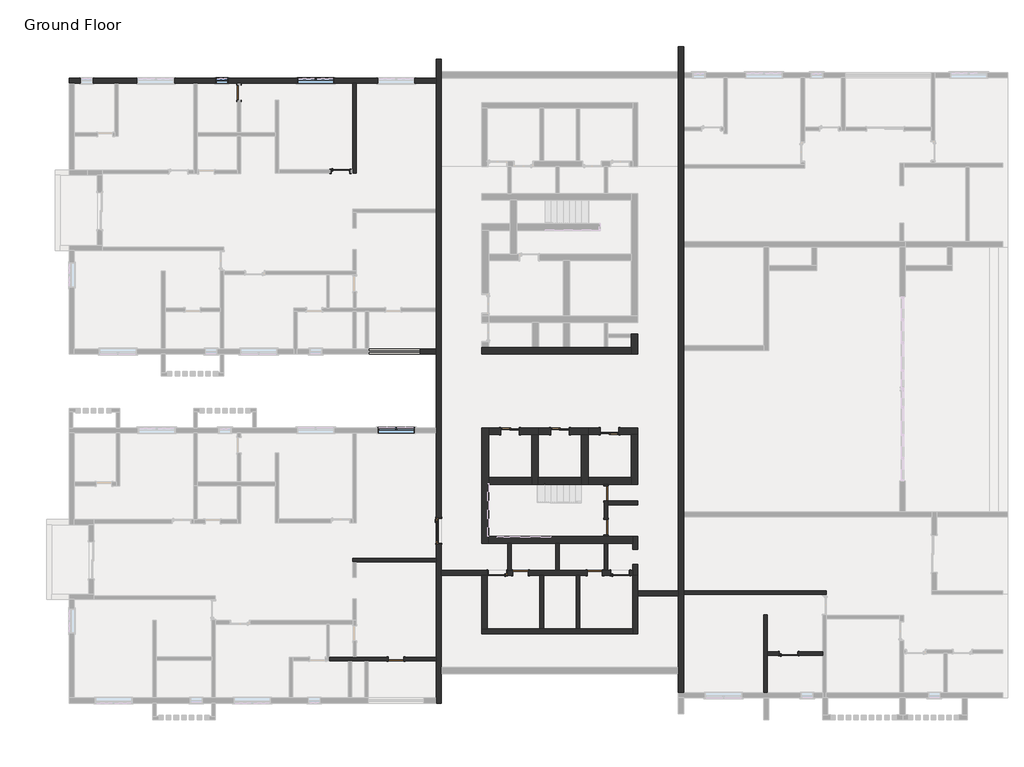
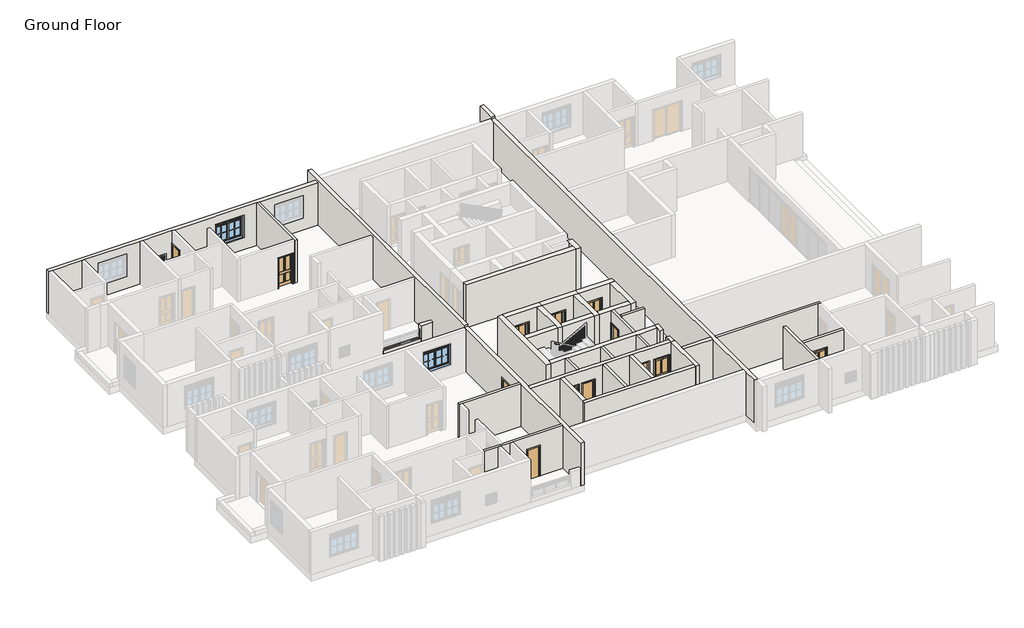
# One storey, part 3 of 9: 37 walls, 14 doors, 3 windows.
# Revit data of these elements (continued)
# Elements 40, 41, 46, 48, 49, 51 (IfcWall, "9\" EXTERIOR WALL") (continued)
#   wall height = 10' - 6"
#   Phase Created = New Construction
#   Base Constraint = Ground Floor
#   Top Constraint = 1st Floor
#   Materials on its faces: "Default Wall", "0 Cream"
# Elements 42, 43, 44, 45 (IfcWall, "9\" EXTERIOR WALL")
#   Top Offset = 0' - 0"
#   Base Offset = 0' - 0"
#   wall height = 10' - 6"
#   Phase Created = New Construction
#   Base Constraint = Ground Floor
#   Top Constraint = 1st Floor
#   Materials on its faces: "0 Cream", "Default Wall"
# Element 47 (IfcWall, "9\" EXTERIOR WALL")
#   Top Offset = 0' - 0"
#   Base Offset = 0' - 0"
#   Unconnected Height = 4' - 0"
#   wall height = 4' - 0"
#   Phase Created = New Construction
#   Base Constraint = Ground Floor
#   Materials on its faces: "Default Wall", "0 Cream"
# Element 50 (IfcWall, "9\" EXTERIOR WALL")
#   Top Offset = 0' - 0"
#   Base Offset = 0' - 0"
#   Unconnected Height = 1' - 0"
#   wall height = 1' - 0"
#   Phase Created = New Construction
#   Base Constraint = Ground Floor
#   Materials on its faces: "Default Wall", "0 Cream"
# Element 52 (IfcWindow, "Window-Casement-Double-Awning-Double : 6' x 5'")
#   Mark = "6"
#   Window Inset = 0' - 0"
#   Interior Wall Closure = 0' - 2 1/4"
#   Frame Extension = 0' - 0 1/4"
#   Exterior Wall Closure = 0' - 1 1/4"
#   Interior Trim Visibility = yes
#   Exterior Trim Visibility = yes
#   Phase Created = New Construction
#   Materials on its faces: "Wood - Stained", "Glass", "Clad - White"
# Element 53 (IfcWindow, "Window-Casement-Double-Awning-Double : 6' x 5'")
#   Mark = "11"
#   Window Inset = 0' - 0"
#   Interior Wall Closure = 0' - 2 1/4"
#   Frame Extension = 0' - 0 1/4"
#   Exterior Wall Closure = 0' - 1 1/4"
#   Interior Trim Visibility = yes
#   Exterior Trim Visibility = yes
#   Phase Created = New Construction
#   Materials on its faces: "Wood - Stained", "Glass", "Clad - White"
# Element 54 (IfcWindow, "Window-Double-Hung")
#   Mark = "14"
#   Window Inset = 0' - 0"
#   Interior Wall Closure = 0' - 1 1/2"
#   Frame Extension = 0' - 1 1/4"
#   Exterior Wall Closure = 0' - 0 1/2"
#   Interior Trim Visibility = yes
#   Indicator Visibility = yes
#   Exterior Trim Visibility = yes
#   Phase Created = New Construction
#   Materials on its faces: "Wood - Stained", "Glass", "Clad - White"
# Materials
#   "Cherry": class "Wood", colour RGB 226 177 128, transparency 0, Description = "Prunus Serotina", Cost = 0
#   "Glass": class "Glass", colour RGB 0 128 192, transparency 0.75, Description = "Soda Lime Glass", Cost = 0
#   "Aluminum": class "Metal", colour RGB 247 247 247, transparency 0, Description = "Aluminum 6061", Cost = 0
#   "Wood - Birch - Solid Stained Light Low Gloss": class "Wood", colour RGB 210 159 95, transparency 0, Cost = 0
#   "Paint - Sienna": colour RGB 118 70 51, transparency 0, Cost = 0
#   "Door - Panel": class "Wood", colour RGB 210 159 95, transparency 0, Cost = 0
#   "Door - Frame": colour RGB 118 70 51, transparency 0, Cost = 0
#   "0 Cream": class "Generic", colour RGB 120 120 120, transparency 0, Cost = 0
#   "Wood - Stained": class "Wood", colour RGB 224 178 126, transparency 0, Cost = 0
#   "Clad - White": class "Wood", colour RGB 242 242 238, transparency 0, Cost = 0
#   "Default Wall": colour RGB 128 128 128, transparency 0, Cost = 0
